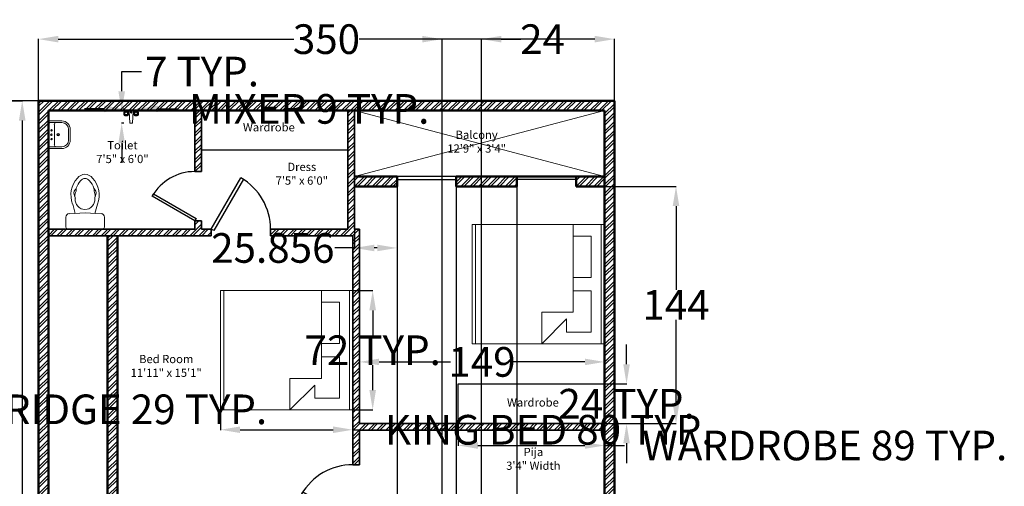
# Model space of a CAD drawing. Units: inches. Extents: x 73 to 1216, y -495 to 328.
# Tile 9 of 9: x 569 to 1167, y 45 to 328. Entities that reach past the tile are written whole.
import ezdxf

# ---------------------------------------------------------------- set-up
doc = ezdxf.new("R2010")
doc.units = ezdxf.units.IN
for name, color, linetype, lineweight in [('A-ANNO-DIMS', 2, 'Continuous', 18), ('A-AREA-IDEN', 7, 'Continuous', 18), ('A-DOOR', 3, 'Continuous', 25), ('A-FLOR-CASE', 2, 'Continuous', 25), ('A-FLOR-FIXT', 9, 'Continuous', 18), ('A-FLOR-OPEN', 8, 'Continuous', 13), ('A-WALL-PATT', 8, 'Continuous', 13), ('Furniture', 2, 'Continuous', 18), ('Inner Walls', 5, 'Continuous', 35), ('Outer Walls', 1, 'Continuous', 50), ('Text-T18', 7, 'Continuous', 18)]:
    doc.layers.add(name, color=color, linetype=linetype, lineweight=lineweight)
doc.styles.get("Standard").update_dxf_attribs({"font": 'arial.ttf'})
doc.dimstyles.get("Standard").update_dxf_attribs({"dimtxt": 18, "dimasz": 12, "dimexe": 0.18, "dimexo": 0.0625, "dimgap": 0.09, "dimtad": 0, "dimtih": 1, "dimtoh": 1, "dimdec": 0, "dimzin": 0, "dimdsep": 46, "dimlunit": 3, "dimtxsty": 'Standard', "dimcen": 0.09, "dimadec": 0, "dimazin": 0, "dimtfac": 1, "dimtdec": 0, "dimtofl": 0, "dimtmove": 0, "dimatfit": 3, "dimfxl": 1, "dimtolj": 1, "dimtzin": 0, "dimarcsym": 0})
pattern_1 = [(45, (-647.324, -1257.0093), (-2.694077, 2.694077), []), (45, (-645.528, -1257.0093), (-2.694077, 2.694077), [])]

# ---------------------------------------------------------------- blocks, each defined once
blk = doc.blocks.new('*U2')
for p, q in [((0, 0), (0, -4)), ((36, 0), (36, -4))]:
    blk.add_line(p, q)
blk.add_lwpolyline([(0, 0), (18, 31.18), (19.52, 30.3), (1.52, -0.88)], close=True)
blk.add_arc((0, 0), 36, 0, 60)
blk = doc.blocks.new('*U3')
for p, q in [((0, 0), (0, -4)), ((30, 0), (30, -4))]:
    blk.add_line(p, q)
blk.add_lwpolyline([(0, 0), (15, 25.98), (16.52, 25.11), (1.52, -0.88)], close=True)
blk.add_arc((0, 0), 30, 0, 60)
blk = doc.blocks.new('*U21')
for p, q in [((0, 0), (0, -6)), ((36, 0), (36, -6))]:
    blk.add_line(p, q)
blk.add_lwpolyline([(0, 0), (36, 0), (36, -1.75), (0, -1.75)], close=True)
blk = doc.blocks.new('KING-00')
for p, q in [((-0.897, -0.947), (-0.897, 0.882)), ((0.602, 0.882), (0.602, -0.464)), ((1.034, -0.947), (1.034, 0.882)), ((0.602, 0.704), (0.881, 0.704)), ((0.881, 0.069), (0.881, 0.704)), ((0.602, 0.069), (0.881, 0.069)), ((0.881, -0.134), (0.602, -0.134)), ((0.881, -0.769), (0.881, -0.134)), ((0.119, -0.464), (0.119, -0.947)), ((0.602, -0.464), (0.119, -0.464)), ((0.119, -0.947), (0.5, -0.566)), ((0.5, -0.769), (0.5, -0.566)), ((0.5, -0.769), (0.881, -0.769))]:
    blk.add_line(p, q)
blk.add_lwpolyline([(-0.948, -0.947), (-0.948, 0.882), (1.084, 0.882), (1.084, -0.947)], close=True)
blk = doc.blocks.new('A$C1308471B')
at = {"ltscale": 20}
for p, q in [((0, 0.461), (0, 0.019)), ((0.035, 0.479), (0.15, 0.479)), ((0.201, 0.24), (0.192, 0.438)), ((0.196, 0.364), (0.311, 0.395)), ((0.498, 0.357), (0.482, 0.371)), ((0.502, 0.353), (0.472, 0.353)), ((0.201, 0.24), (0.192, 0.041)), ((0.502, 0.13), (0.472, 0.13)), ((0.498, 0.126), (0.482, 0.112)), ((0.035, 0), (0.15, 0)), ((0.196, 0.119), (0.311, 0.088))]:
    blk.add_line(p, q, dxfattribs=at)
for centre, radius, start, end in [((0.006, 0.461), 0.006, 136.5269, 180), ((0.035, 0.433), 0.0465, 90, 136.5269), ((0.15, 0.436), 0.0429, 2.5755, 90), ((0.425, 0.11), 0.307, 47.4135, 111.7924), ((0.449, 0.264), 0.115, 79.3968, 118.5742), ((0.405, 0.216), 0.153, 63.502, 90.4522), ((0.466, 0.351), 0.0255, 50, 79.3968), ((0.365, 0.242), 0.121, 83.3523, 180), ((0.382, 0.387), 0.0255, 263.3523, 298.5742), ((0.515, 0.377), 0.0255, 230, 251.3881), ((0.502, 0.327), 0.0255, 70.3751, 90), ((0.425, 0.11), 0.256, 46.612, 70.3751), ((0.565, 0.242), 0.065, 0, 57.2974), ((0.565, 0.242), 0.116, 0, 54.7115), ((0.365, 0.242), 0.121, 180, 276.6477), ((0.425, 0.373), 0.307, 248.2076, 312.5865), ((0.405, 0.267), 0.153, 269.5478, 296.498), ((0.515, 0.106), 0.0255, 108.6119, 130), ((0.502, 0.156), 0.0255, 270, 289.6249), ((0.425, 0.373), 0.256, 289.6249, 313.388), ((0.565, 0.242), 0.065, 302.7026, 0), ((0.565, 0.242), 0.116, 305.2885, 0), ((0.006, 0.019), 0.006, 180, 223.4731), ((0.035, 0.047), 0.0465, 223.4731, 270), ((0.15, 0.043), 0.0429, 270, 357.4245), ((0.382, 0.096), 0.0255, 61.4258, 96.6477), ((0.449, 0.22), 0.115, 241.4258, 280.6032), ((0.466, 0.132), 0.0255, 280.6032, 310)]:
    blk.add_arc(centre, radius, start, end, dxfattribs=at)
blk = doc.blocks.new('A$C57EA129C')
for p, q in [((0, 0.443), (0, 0.178)), ((0.016, 0.459), (0.563, 0.459)), ((0.036, 0.432), (0.036, 0.29)), ((0.045, 0.441), (0.535, 0.441)), ((0.544, 0.432), (0.544, 0.29)), ((0.579, 0.443), (0.579, 0.178)), ((0.036, 0.29), (0.036, 0.178)), ((0.08, 0.334), (0.499, 0.334)), ((0.544, 0.29), (0.544, 0.178)), ((0.178, 0.036), (0.401, 0.036)), ((0.178, 0), (0.401, 0))]:
    blk.add_line(p, q)
for centre, radius in [((0.198, 0.392), 0.0143), ((0.29, 0.255), 0.0267), ((0.29, 0.255), 0.0178), ((0.29, 0.396), 0.0156), ((0.381, 0.392), 0.0143)]:
    blk.add_circle(centre, radius)
for centre, radius, start, end in [((0.016, 0.443), 0.016, 90, 180), ((0.045, 0.432), 0.00891, 90, 180), ((0.535, 0.432), 0.00891, 0, 90), ((0.563, 0.443), 0.016, 0, 90), ((0.08, 0.29), 0.0445, 90, 180), ((0.499, 0.29), 0.0445, 0, 90), ((0.178, 0.178), 0.178, 180, 270), ((0.178, 0.178), 0.143, 180, 270), ((0.401, 0.178), 0.178, 270, 0), ((0.401, 0.178), 0.143, 270, 0)]:
    blk.add_arc(centre, radius, start, end)
blk = doc.blocks.new('A$C68D75330')
for p, q in [((0.155, 0.406), (0.155, 0.451)), ((0.167, 0.404), (0.167, 0.454)), ((0.172, 0.459), (0.222, 0.459)), ((0.222, 0.399), (0.172, 0.399)), ((0.175, 0.471), (0.22, 0.471)), ((0.22, 0.386), (0.175, 0.386)), ((0.227, 0.454), (0.227, 0.404)), ((0.24, 0.451), (0.24, 0.406)), ((0.264, 0.256), (0.252, 0.461)), ((0.275, 0.471), (0.305, 0.471)), ((0.327, 0.461), (0.315, 0.256)), ((0.34, 0.451), (0.34, 0.406)), ((0.352, 0.454), (0.352, 0.404)), ((0.407, 0.459), (0.357, 0.459)), ((0.357, 0.399), (0.407, 0.399)), ((0.405, 0.471), (0.36, 0.471)), ((0.36, 0.386), (0.405, 0.386)), ((0.412, 0.404), (0.412, 0.454)), ((0.425, 0.406), (0.425, 0.451)), ((0.306, 0.246), (0.274, 0.246))]:
    blk.add_line(p, q)
for centre, radius in [((0.197, 0.429), 0.03), ((0.197, 0.429), 0.0232), ((0.29, 0.446), 0.0125), ((0.29, 0.446), 0.00625), ((0.382, 0.429), 0.03), ((0.382, 0.429), 0.0232)]:
    blk.add_circle(centre, radius)
for centre, radius, start, end in [((0.175, 0.451), 0.02, 90, 180), ((0.175, 0.406), 0.02, 180, 270), ((0.172, 0.454), 0.005, 90, 180), ((0.172, 0.404), 0.005, 180, 270), ((0.22, 0.451), 0.02, 0, 90), ((0.22, 0.406), 0.02, 270, 0), ((0.222, 0.454), 0.005, 0, 90), ((0.222, 0.404), 0.005, 270, 0), ((0.274, 0.444), 0.0273, 87.1975, 140.7274), ((0.306, 0.444), 0.0273, 39.2726, 92.8025), ((0.36, 0.451), 0.02, 90, 180), ((0.36, 0.406), 0.02, 180, 270), ((0.357, 0.454), 0.005, 90, 180), ((0.357, 0.404), 0.005, 180, 270), ((0.405, 0.451), 0.02, 0, 90), ((0.405, 0.406), 0.02, 270, 0), ((0.407, 0.454), 0.005, 0, 90), ((0.407, 0.404), 0.005, 270, 0), ((0.274, 0.256), 0.01, 183.3274, 270), ((0.306, 0.256), 0.01, 270, 356.6726)]:
    blk.add_arc(centre, radius, start, end)
blk = doc.blocks.new('WARDROBE-89X24')
blk.add_lwpolyline([(0, 24), (89, 24), (89, 0), (0, 0)], close=True)
blk = doc.blocks.new('*D26')
at = {"layer": 'A-ANNO-DIMS', "color": 0, "lineweight": -2, "transparency": 16777216}
for p, q in [((690.69, 91.4), (690.69, 79.21)), ((771.16, 91.4), (771.16, 79.21)), ((702.69, 79.39), (759.16, 79.39)), ((771.16, 79.39), (783.16, 79.39))]:
    blk.add_line(p, q, dxfattribs=at)
at = {"layer": 'A-ANNO-DIMS', "color": 0, "transparency": 16777216}
for points in [[(702.69, 81.39), (702.69, 77.39), (690.69, 79.39)], [(759.16, 81.39), (759.16, 77.39), (771.16, 79.39)]]:
    blk.add_solid(points, dxfattribs=at)
at = {"layer": 'Defpoints', "color": 0, "transparency": 16777216}
for p in [(690.69, 91.46), (771.16, 91.46), (771.16, 79.39)]:
    blk.add_point(p, dxfattribs=at)
at = {"layer": 'A-ANNO-DIMS', "color": 0, "transparency": 16777216, "insert": (890.24, 79.39), "char_height": 18, "attachment_point": 5}
blk.add_mtext('\\A1;KING BED 80 TYP.', dxfattribs=at)
blk = doc.blocks.new('*D27')
at = {"layer": 'A-ANNO-DIMS', "color": 0, "lineweight": -2, "transparency": 16777216}
for p, q in [((771.23, 163.89), (783.42, 163.89)), ((783.24, 151.89), (783.24, 136.81)), ((783.24, 103.46), (783.24, 118.54)), ((771.23, 91.46), (783.42, 91.46))]:
    blk.add_line(p, q, dxfattribs=at)
at = {"layer": 'A-ANNO-DIMS', "color": 0, "transparency": 16777216}
for points in [[(781.24, 151.89), (785.24, 151.89), (783.24, 163.89)], [(781.24, 103.46), (785.24, 103.46), (783.24, 91.46)]]:
    blk.add_solid(points, dxfattribs=at)
at = {"layer": 'Defpoints', "color": 0, "transparency": 16777216}
for p in [(771.16, 163.89), (783.24, 163.89), (771.16, 91.46)]:
    blk.add_point(p, dxfattribs=at)
at = {"layer": 'A-ANNO-DIMS', "color": 0, "transparency": 16777216, "insert": (783.24, 127.68), "char_height": 18, "attachment_point": 5}
blk.add_mtext('\\A1;72 TYP.', dxfattribs=at)
blk = doc.blocks.new('*D34')
at = {"layer": 'A-ANNO-DIMS', "color": 0, "lineweight": -2, "transparency": 16777216}
for p, q in [((620.04, 274.23), (608.04, 274.23)), ((632.04, 272.97), (632.04, 274.41)), ((640.86, 272.97), (640.86, 274.41)), ((652.86, 274.23), (664.86, 274.23))]:
    blk.add_line(p, q, dxfattribs=at)
at = {"layer": 'A-ANNO-DIMS', "color": 0, "transparency": 16777216}
for points in [[(620.04, 276.23), (620.04, 272.23), (632.04, 274.23)], [(652.86, 276.23), (652.86, 272.23), (640.86, 274.23)]]:
    blk.add_solid(points, dxfattribs=at)
at = {"layer": 'Defpoints', "color": 0, "transparency": 16777216}
for p in [(632.04, 272.9), (640.86, 274.23), (640.86, 272.9)]:
    blk.add_point(p, dxfattribs=at)
at = {"layer": 'A-ANNO-DIMS', "color": 0, "transparency": 16777216, "insert": (744.67, 274.23), "char_height": 18, "attachment_point": 5}
blk.add_mtext('\\A1;MIXER 9 TYP.', dxfattribs=at)
blk = doc.blocks.new('*D35')
at = {"layer": 'A-ANNO-DIMS', "color": 0, "lineweight": -2, "transparency": 16777216}
for p, q in [((630.72, 284.9), (630.72, 296.9)), ((630.72, 296.9), (642.72, 296.9)), ((631.98, 272.9), (630.54, 272.9)), ((631.98, 265.54), (630.54, 265.54)), ((630.72, 253.54), (630.72, 241.54))]:
    blk.add_line(p, q, dxfattribs=at)
at = {"layer": 'A-ANNO-DIMS', "color": 0, "transparency": 16777216}
for points in [[(628.72, 284.9), (632.72, 284.9), (630.72, 272.9)], [(628.72, 253.54), (632.72, 253.54), (630.72, 265.54)]]:
    blk.add_solid(points, dxfattribs=at)
at = {"layer": 'Defpoints', "color": 0, "transparency": 16777216}
for p in [(630.72, 272.9), (632.04, 272.9), (632.04, 265.54)]:
    blk.add_point(p, dxfattribs=at)
at = {"layer": 'A-ANNO-DIMS', "color": 0, "transparency": 16777216, "insert": (679.55, 296.9), "char_height": 18, "attachment_point": 5}
blk.add_mtext('\\A1;7 TYP.', dxfattribs=at)
blk = doc.blocks.new('*D38')
at = {"layer": 'A-ANNO-DIMS', "color": 0, "lineweight": -2, "transparency": 16777216}
for p, q in [((835.16, 83.11), (835.16, 69.65)), ((924.16, 83.11), (924.16, 69.65)), ((847.16, 69.83), (912.16, 69.83)), ((924.16, 69.83), (936.16, 69.83))]:
    blk.add_line(p, q, dxfattribs=at)
at = {"layer": 'A-ANNO-DIMS', "color": 0, "transparency": 16777216}
for points in [[(847.16, 71.83), (847.16, 67.83), (835.16, 69.83)], [(912.16, 71.83), (912.16, 67.83), (924.16, 69.83)]]:
    blk.add_solid(points, dxfattribs=at)
at = {"layer": 'Defpoints', "color": 0, "transparency": 16777216}
for p in [(835.16, 83.18), (924.16, 83.18), (924.16, 69.83)]:
    blk.add_point(p, dxfattribs=at)
at = {"layer": 'A-ANNO-DIMS', "color": 0, "transparency": 16777216, "insert": (1057.97, 69.83), "char_height": 18, "attachment_point": 5}
blk.add_mtext('\\A1;WARDROBE 89 TYP.', dxfattribs=at)
blk = doc.blocks.new('*D39')
at = {"layer": 'A-ANNO-DIMS', "color": 0, "lineweight": -2, "transparency": 16777216}
for p, q in [((937.51, 119.18), (937.51, 131.18)), ((924.23, 107.18), (937.69, 107.18)), ((924.23, 83.18), (937.69, 83.18)), ((937.51, 71.18), (937.51, 59.18))]:
    blk.add_line(p, q, dxfattribs=at)
at = {"layer": 'A-ANNO-DIMS', "color": 0, "transparency": 16777216}
for points in [[(935.51, 119.18), (939.51, 119.18), (937.51, 107.18)], [(935.51, 71.18), (939.51, 71.18), (937.51, 83.18)]]:
    blk.add_solid(points, dxfattribs=at)
at = {"layer": 'Defpoints', "color": 0, "transparency": 16777216}
for p in [(924.16, 107.18), (937.51, 107.18), (924.16, 83.18)]:
    blk.add_point(p, dxfattribs=at)
at = {"layer": 'A-ANNO-DIMS', "color": 0, "transparency": 16777216, "insert": (937.51, 95.18), "char_height": 18, "attachment_point": 5}
blk.add_mtext('\\A1;24 TYP.', dxfattribs=at)
blk = doc.blocks.new('*D40')
at = {"layer": 'A-ANNO-DIMS', "color": 0, "lineweight": -2, "transparency": 16777216}
for p, q in [((497.66, 96.03), (497.66, 91.62)), ((526.23, 96.03), (526.23, 91.62)), ((509.66, 91.8), (514.23, 91.8)), ((526.23, 91.8), (538.23, 91.8))]:
    blk.add_line(p, q, dxfattribs=at)
at = {"layer": 'A-ANNO-DIMS', "color": 0, "transparency": 16777216}
for points in [[(509.66, 93.8), (509.66, 89.8), (497.66, 91.8)], [(514.23, 93.8), (514.23, 89.8), (526.23, 91.8)]]:
    blk.add_solid(points, dxfattribs=at)
at = {"layer": 'Defpoints', "color": 0, "transparency": 16777216}
for p in [(497.66, 96.09), (526.23, 96.09), (526.23, 91.8)]:
    blk.add_point(p, dxfattribs=at)
at = {"layer": 'A-ANNO-DIMS', "color": 0, "transparency": 16777216, "insert": (632.61, 91.8), "char_height": 18, "attachment_point": 5}
blk.add_mtext('\\A1;FRIDGE 29 TYP.', dxfattribs=at)
blk = doc.blocks.new('*D51')
at = {"layer": 'A-ANNO-DIMS', "color": 0, "lineweight": -2, "transparency": 16777216}
for p, q in [((532.94, 279.18), (570.45, 279.18)), ((570.27, 267.18), (570.27, -65.04)), ((570.27, -415.82), (570.27, -83.6)), ((532.94, -427.82), (570.45, -427.82))]:
    blk.add_line(p, q, dxfattribs=at)
at = {"layer": 'A-ANNO-DIMS', "color": 0, "transparency": 16777216}
for points in [[(568.27, 267.18), (572.27, 267.18), (570.27, 279.18)], [(568.27, -415.82), (572.27, -415.82), (570.27, -427.82)]]:
    blk.add_solid(points, dxfattribs=at)
at = {"layer": 'Defpoints', "color": 0, "transparency": 16777216}
for p in [(532.87, 279.18), (570.27, 279.18), (532.87, -427.82)]:
    blk.add_point(p, dxfattribs=at)
at = {"layer": 'A-ANNO-DIMS', "color": 0, "transparency": 16777216, "insert": (570.27, -74.32), "char_height": 18, "attachment_point": 5}
blk.add_mtext('\\A1;707', dxfattribs=at)
blk = doc.blocks.new('*D52')
at = {"layer": 'A-ANNO-DIMS', "color": 0, "lineweight": -2, "transparency": 16777216}
for p, q in [((580.16, 279.24), (580.16, 316.76)), ((592.16, 316.58), (735.23, 316.58)), ((918.16, 316.58), (775.1, 316.58)), ((930.16, 279.24), (930.16, 316.76))]:
    blk.add_line(p, q, dxfattribs=at)
at = {"layer": 'A-ANNO-DIMS', "color": 0, "transparency": 16777216}
for points in [[(592.16, 318.58), (592.16, 314.58), (580.16, 316.58)], [(918.16, 318.58), (918.16, 314.58), (930.16, 316.58)]]:
    blk.add_solid(points, dxfattribs=at)
at = {"layer": 'Defpoints', "color": 0, "transparency": 16777216}
for p in [(930.16, 316.58), (580.16, 279.18), (930.16, 279.18)]:
    blk.add_point(p, dxfattribs=at)
at = {"layer": 'A-ANNO-DIMS', "color": 0, "transparency": 16777216, "insert": (755.16, 316.58), "char_height": 18, "attachment_point": 5}
blk.add_mtext('\\A1;350', dxfattribs=at)
blk = doc.blocks.new('*D53')
at = {"layer": 'A-ANNO-DIMS', "color": 0, "lineweight": -2, "transparency": 16777216}
for p, q in [((580.1, 279.18), (542.58, 279.18)), ((542.76, 267.18), (542.76, -65.04)), ((542.76, -415.82), (542.76, -83.6)), ((580.1, -427.82), (542.58, -427.82))]:
    blk.add_line(p, q, dxfattribs=at)
at = {"layer": 'A-ANNO-DIMS', "color": 0, "transparency": 16777216}
for points in [[(540.76, 267.18), (544.76, 267.18), (542.76, 279.18)], [(540.76, -415.82), (544.76, -415.82), (542.76, -427.82)]]:
    blk.add_solid(points, dxfattribs=at)
at = {"layer": 'Defpoints', "color": 0, "transparency": 16777216}
for p in [(542.76, 279.18), (580.16, 279.18), (580.16, -427.82)]:
    blk.add_point(p, dxfattribs=at)
at = {"layer": 'A-ANNO-DIMS', "color": 0, "transparency": 16777216, "insert": (542.76, -74.32), "char_height": 18, "attachment_point": 5}
blk.add_mtext('\\A1;707', dxfattribs=at)
blk = doc.blocks.new('*D57')
at = {"layer": 'A-ANNO-DIMS', "color": 0, "lineweight": -2, "transparency": 16777216}
for p, q in [((775.16, 83.24), (775.16, 120.76)), ((787.16, 120.58), (830.52, 120.58)), ((912.16, 120.58), (868.81, 120.58)), ((924.16, 83.24), (924.16, 120.76))]:
    blk.add_line(p, q, dxfattribs=at)
at = {"layer": 'A-ANNO-DIMS', "color": 0, "transparency": 16777216}
for points in [[(787.16, 122.58), (787.16, 118.58), (775.16, 120.58)], [(912.16, 122.58), (912.16, 118.58), (924.16, 120.58)]]:
    blk.add_solid(points, dxfattribs=at)
at = {"layer": 'Defpoints', "color": 0, "transparency": 16777216}
for p in [(924.16, 120.58), (775.16, 83.18), (924.16, 83.18)]:
    blk.add_point(p, dxfattribs=at)
at = {"layer": 'A-ANNO-DIMS', "color": 0, "transparency": 16777216, "insert": (849.66, 120.58), "char_height": 18, "attachment_point": 5}
blk.add_mtext('\\A1;149', dxfattribs=at)
blk = doc.blocks.new('*D58')
at = {"layer": 'A-ANNO-DIMS', "color": 0, "lineweight": -2, "transparency": 16777216}
for p, q in [((924.23, 227.18), (967.74, 227.18)), ((967.56, 215.18), (967.56, 164.3)), ((967.56, 95.18), (967.56, 146.05)), ((924.23, 83.18), (967.74, 83.18))]:
    blk.add_line(p, q, dxfattribs=at)
at = {"layer": 'A-ANNO-DIMS', "color": 0, "transparency": 16777216}
for points in [[(965.56, 215.18), (969.56, 215.18), (967.56, 227.18)], [(965.56, 95.18), (969.56, 95.18), (967.56, 83.18)]]:
    blk.add_solid(points, dxfattribs=at)
at = {"layer": 'Defpoints', "color": 0, "transparency": 16777216}
for p in [(924.16, 227.18), (967.56, 227.18), (924.16, 83.18)]:
    blk.add_point(p, dxfattribs=at)
at = {"layer": 'A-ANNO-DIMS', "color": 0, "transparency": 16777216, "insert": (967.56, 155.18), "char_height": 18, "attachment_point": 5}
blk.add_mtext('\\A1;144', dxfattribs=at)
blk = doc.blocks.new('*D67')
at = {"layer": 'A-ANNO-DIMS', "color": 0, "lineweight": -2, "transparency": 16777216}
for p, q in [((798.02113, 227.113801), (798.02113, -465.403699)), ((834.02113, 227.113801), (834.02113, -465.403699)), ((786.02113, -465.223699), (774.02113, -465.223699)), ((846.02113, -465.223699), (858.02113, -465.223699))]:
    blk.add_line(p, q, dxfattribs=at)
at = {"layer": 'A-ANNO-DIMS', "color": 0, "transparency": 16777216}
for points in [[(786.02113, -463.223699), (786.02113, -467.223699), (798.02113, -465.223699)], [(846.02113, -463.223699), (846.02113, -467.223699), (834.02113, -465.223699)]]:
    blk.add_solid(points, dxfattribs=at)
at = {"layer": 'Defpoints', "color": 0, "transparency": 16777216}
for p in [(798.02113, 227.176301), (834.02113, 227.176301), (834.02113, -465.223699)]:
    blk.add_point(p, dxfattribs=at)
at = {"layer": 'A-ANNO-DIMS', "color": 0, "transparency": 16777216, "insert": (816.02113, -465.223699), "char_height": 18, "attachment_point": 5}
blk.add_mtext('\\A1;36', dxfattribs=at)
blk = doc.blocks.new('*D68')
at = {"layer": 'A-ANNO-DIMS', "color": 0, "lineweight": -2, "transparency": 16777216}
for p, q in [((834.02, 227.11), (834.02, -465.4)), ((870.82, 227.11), (870.82, -465.4)), ((846.02, -465.22), (858.82, -465.22)), ((870.82, -465.22), (882.82, -465.22))]:
    blk.add_line(p, q, dxfattribs=at)
at = {"layer": 'A-ANNO-DIMS', "color": 0, "transparency": 16777216}
for points in [[(846.02, -463.22), (846.02, -467.22), (834.02, -465.22)], [(858.82, -463.22), (858.82, -467.22), (870.82, -465.22)]]:
    blk.add_solid(points, dxfattribs=at)
at = {"layer": 'Defpoints', "color": 0, "transparency": 16777216}
for p in [(834.02, 227.18), (870.82, 227.18), (870.82, -465.22)]:
    blk.add_point(p, dxfattribs=at)
at = {"layer": 'A-ANNO-DIMS', "color": 0, "transparency": 16777216, "insert": (906.3, -465.22), "char_height": 18, "attachment_point": 5}
blk.add_mtext('\\A1;36.8', dxfattribs=at)
blk = doc.blocks.new('*D69')
at = {"layer": 'A-ANNO-DIMS', "color": 0, "lineweight": -2, "transparency": 16777216}
for p, q in [((772.16, 227.11), (772.16, 189.6)), ((798.02, 227.11), (798.02, 189.6)), ((772.16, 189.78), (760.16, 189.78)), ((786.02, 189.78), (784.16, 189.78))]:
    blk.add_line(p, q, dxfattribs=at)
at = {"layer": 'A-ANNO-DIMS', "color": 0, "transparency": 16777216}
for points in [[(784.16, 191.78), (784.16, 187.78), (772.16, 189.78)], [(786.02, 191.78), (786.02, 187.78), (798.02, 189.78)]]:
    blk.add_solid(points, dxfattribs=at)
at = {"layer": 'Defpoints', "color": 0, "transparency": 16777216}
for p in [(772.16, 227.18), (798.02, 227.18), (772.16, 189.78)]:
    blk.add_point(p, dxfattribs=at)
at = {"layer": 'A-ANNO-DIMS', "color": 0, "transparency": 16777216, "insert": (722.56, 189.78), "char_height": 18, "attachment_point": 5}
blk.add_mtext('\\A1;25.856', dxfattribs=at)
blk = doc.blocks.new('*D77')
at = {"layer": 'A-ANNO-DIMS', "color": 0, "lineweight": -2, "transparency": 16777216}
for p, q in [((813.36, 316.58), (801.36, 316.58)), ((825.36, -180.08), (825.36, 316.76)), ((849.36, -180.08), (849.36, 316.76)), ((861.36, 316.58), (873.36, 316.58))]:
    blk.add_line(p, q, dxfattribs=at)
at = {"layer": 'A-ANNO-DIMS', "color": 0, "transparency": 16777216}
for points in [[(813.36, 318.58), (813.36, 314.58), (825.36, 316.58)], [(861.36, 318.58), (861.36, 314.58), (849.36, 316.58)]]:
    blk.add_solid(points, dxfattribs=at)
at = {"layer": 'Defpoints', "color": 0, "transparency": 16777216}
for p in [(849.36, 316.58), (825.36, -180.14), (849.36, -180.14)]:
    blk.add_point(p, dxfattribs=at)
at = {"layer": 'A-ANNO-DIMS', "color": 0, "transparency": 16777216, "insert": (886.46, 316.58), "char_height": 18, "attachment_point": 5}
blk.add_mtext('\\A1;24', dxfattribs=at)

msp = doc.modelspace()

# ---------------------------------------------------------------- hatches: boundary and pattern name
at = {"layer": 'A-WALL-PATT'}
h = msp.add_hatch(dxfattribs=at)
h.set_pattern_fill('ANSI32', color=256, scale=0.4)
h.set_pattern_definition(pattern_1)
h.paths.add_polyline_path([(586.1647, 273.1763), (924.1647, 273.1763), (924.1647, -421.8237), (753.1647, -421.8237), (753.1647, -427.8237), (930.1647, -427.8237), (930.1647, 279.1763), (580.1647, 279.1763), (580.1647, -427.8237), (633.1647, -427.8237), (633.1647, -421.8237), (586.1647, -421.8237)])
h = msp.add_hatch(dxfattribs=at)
h.set_pattern_fill('ANSI32', color=256, scale=0.4)
h.set_pattern_definition(pattern_1)
h.paths.add_polyline_path([(685.1647, 201.1763), (679.1647, 201.1763), (679.1647, 206.1763), (675.1647, 206.1763), (675.1647, 201.1763), (586.1647, 201.1763), (586.1647, 197.1763), (685.1647, 197.1763)])
h.paths.add_polyline_path([(679.1647, 273.1763), (675.1647, 273.1763), (675.1647, 236.1763), (679.1647, 236.1763)])
h.paths.add_polyline_path([(775.1647, 201.1763), (772.1647, 201.1763), (772.1647, 273.1763), (768.1647, 273.1763), (768.1647, 249.1763), (768.1647, 201.1763), (721.1647, 201.1763), (721.1647, 197.1763), (771.1647, 197.1763), (771.1647, 58.1763), (775.1647, 58.1763)])
h.paths.add_polyline_path([(798.0211, 233.1763), (772.1647, 233.1763), (772.1647, 227.1763), (798.0211, 227.1763)])
h.paths.add_polyline_path([(870.8232, 233.1763), (834.0211, 233.1763), (834.0211, 227.1763), (870.8232, 227.1763)])
h.paths.add_polyline_path([(924.1647, 233.1763), (906.8232, 233.1763), (906.8232, 227.1763), (924.1647, 227.1763)])
h.paths.add_polyline_path([(924.1647, 83.1763), (775.1647, 83.1763), (775.1647, 79.1763), (924.1647, 79.1763)])
h.paths.add_polyline_path([(775.1647, 22.1763), (771.1647, 22.1763), (771.1647, 16.1763), (628.1647, 16.1763), (628.1647, 12.1763), (775.1647, 12.1763)])
h.paths.add_polyline_path([(692.1647, 12.1763), (688.1647, 12.1763), (688.1647, -52.8237), (692.1647, -52.8237)])
h.paths.add_polyline_path([(924.1647, 39.1763), (824.1647, 39.1763), (824.1647, 35.1763), (924.1647, 35.1763)])
h.paths.add_polyline_path([(874.6647, -29.8237), (864.1647, -29.8237), (824.1647, -29.8237), (824.1647, -87.8237), (817.1647, -87.8237), (817.1647, -91.8237), (844.6647, -91.8237), (844.6647, -87.8237), (828.1647, -87.8237), (828.1647, -33.8237), (874.6647, -33.8237)])
h.paths.add_polyline_path([(924.1647, -29.8237), (910.6647, -29.8237), (910.6647, -33.8237), (924.1647, -33.8237)])
h.paths.add_polyline_path([(924.1647, -87.8237), (904.6647, -87.8237), (904.6647, -91.8237), (924.1647, -91.8237)])
h.paths.add_polyline_path([(777.1647, -88.8237), (761.1647, -88.8237), (761.1647, -92.8237), (767.1647, -92.8237), (767.1647, -224.8237), (771.1647, -224.8237), (771.1647, -92.8237), (777.1647, -92.8237)])
h.paths.add_polyline_path([(725.1647, -88.8237), (628.1647, -88.8237), (628.1647, -92.8237), (725.1647, -92.8237)])
h.paths.add_polyline_path([(692.1647, -82.8237), (688.1647, -82.8237), (688.1647, -88.8237), (692.1647, -88.8237)])
h.paths.add_polyline_path([(767.1647, -313.8237), (924.1647, -313.8237), (924.1647, -307.8237), (763.1647, -307.8237), (763.1647, -421.8237), (767.1647, -421.8237)])
h = msp.add_hatch(dxfattribs=at)
h.set_pattern_fill('ANSI32', color=256, scale=0.4)
h.set_pattern_definition(pattern_1)
h.paths.add_polyline_path([(628.1647, 197.1763), (622.1647, 197.1763), (622.1647, -230.8237), (771.1647, -230.8237), (771.1647, -224.8237), (628.1647, -224.8237)])

# ---------------------------------------------------------------- linework, layer by layer
at = {"layer": 'A-FLOR-OPEN'}
for p, q in [((924.1647, 233.1763), (772.1647, 273.1763)), ((772.1647, 233.1763), (924.1647, 273.1763))]:
    msp.add_line(p, q, dxfattribs=at)
at = {"layer": 'Inner Walls'}
for p, q in [((675.1647, 273.1763), (675.1647, 236.1763)), ((679.1647, 273.1763), (679.1647, 236.1763)), ((768.1647, 273.1763), (768.1647, 201.1763)), ((772.1647, 273.1763), (772.1647, 201.1763)), ((675.1647, 236.1763), (679.1647, 236.1763)), ((675.1647, 206.1763), (675.1647, 201.1763)), ((679.1647, 206.1763), (675.1647, 206.1763)), ((679.1647, 206.1763), (679.1647, 201.1763)), ((675.1647, 201.1763), (586.1647, 201.1763)), ((685.1647, 201.1763), (679.1647, 201.1763)), ((685.1647, 201.1763), (685.1647, 197.1763)), ((768.1647, 201.1763), (721.1647, 201.1763)), ((721.1647, 197.1763), (721.1647, 201.1763)), ((772.1647, 201.1763), (775.1647, 201.1763)), ((775.1647, 201.1763), (775.1647, 83.1763)), ((685.1647, 197.1763), (586.1647, 197.1763)), ((771.1647, 197.1763), (721.1647, 197.1763)), ((771.1647, 197.1763), (771.1647, 58.1763)), ((775.1647, 83.1763), (924.1647, 83.1763)), ((775.1647, 79.1763), (924.1647, 79.1763)), ((775.1647, 79.1763), (775.1647, 58.1763)), ((775.1647, 58.1763), (771.1647, 58.1763))]:
    msp.add_line(p, q, dxfattribs=at)
at = {"layer": 'Outer Walls'}
for p, q in [((580.1647, 279.1763), (930.1647, 279.1763)), ((580.1647, -427.8237), (580.1647, 279.1763)), ((930.1647, -427.8237), (930.1647, 279.1763)), ((586.1647, 273.1763), (924.1647, 273.1763)), ((586.1647, -421.8237), (586.1647, 273.1763)), ((924.1647, -421.8237), (924.1647, 273.1763)), ((772.1647, 233.1763), (798.0211, 233.1763)), ((798.0211, 233.1763), (798.0211, 227.1763)), ((834.0211, 233.1763), (924.1647, 233.1763)), ((834.0211, 233.1763), (834.0211, 227.1763)), ((870.8232, 233.1763), (870.8232, 227.1763)), ((906.8232, 233.1763), (906.8232, 227.1763)), ((772.1647, 227.1763), (798.0211, 227.1763)), ((834.0211, 227.1763), (870.8232, 227.1763)), ((906.8232, 227.1763), (924.1647, 227.1763)), ((622.1647, -230.8237), (622.1647, 197.1763)), ((628.1647, -224.8237), (628.1647, 197.1763))]:
    msp.add_line(p, q, dxfattribs=at)

# ---------------------------------------------------------------- block references
at = {"layer": 'A-DOOR', "rotation": 90}
for name, p in [('*U3', (675.1647, 206.1763)), ('*U2', (771.1647, 22.1763))]:
    msp.add_blockref(name, p, dxfattribs=at)
at = {"layer": 'A-DOOR'}
for name, p in [('*U2', (685.1647, 201.1763)), ('*U21', (870.8232, 233.1763))]:
    msp.add_blockref(name, p, dxfattribs=at)
at = {"layer": 'A-DOOR', "xscale": -1}
msp.add_blockref('*U21', (834.0211, 233.1763), dxfattribs=at)
at = {"layer": 'A-FLOR-CASE'}
for p in [(679.1651, 249.176), (835.1651, 83.176)]:
    msp.add_blockref('WARDROBE-89X24', p, dxfattribs=at)
at = {"layer": 'A-FLOR-FIXT', "xscale": 32.67217261962217, "yscale": 32.67217261962217, "zscale": 32.67217261962217}
msp.add_blockref('A$C68D75330', (626.9766, 257.4873), dxfattribs=at)
at = {"layer": 'A-FLOR-FIXT'}
for name, p, xscale, yscale, zscale, rotation in [('A$C57EA129C', (599.4641, 266.948), -28.98333223671166, 28.98333223671166, 28.98333223671166, 90), ('A$C1308471B', (620.2612, 201.1763), 48.95497407897215, 48.95497407897215, 48.95497407897215, 89.99999999999996)]:
    msp.add_blockref(name, p, dxfattribs=dict(at, xscale=xscale, yscale=yscale, zscale=zscale, rotation=rotation))
at = {"layer": 'Furniture', "xscale": 39.60249106241186, "yscale": 39.60249106241186, "zscale": 39.60249106241186}
for p in [(881.2158, 169.0885), (728.2158, 128.9661)]:
    msp.add_blockref('KING-00', p, dxfattribs=at)

# ---------------------------------------------------------------- texts
at = {"layer": 'A-AREA-IDEN', "char_height": 5, "attachment_point": 3}
for s, width, insert in [('\\pxqc;{\\fTimes New Roman|b0|i0|c0|p18;Balcony\\P12\'9" x 3\'4"}', 37.203385, (865.0165, 261.0024)), ('\\pxqc;{\\fTimes New Roman|b0|i0|c0|p18;Toilet\\P7\'5" x 6\'0"}', 37.203385, (649.7732, 254.6536)), ('\\pxqc;{\\fTimes New Roman|b0|i0|c0|p18;Dress\\P7\'5" x 6\'0"}', 37.203385, (758.7688, 241.5333)), ('\\pxqc;{\\fTimes New Roman|b0|i0|c0|p18;Bed Room\\P11\'11" x 15\'1"}', 44.177391, (679.8534, 124.8296)), ('\\pxqc;{\\fTimes New Roman|b0|i0|c0|p18;Pija\\P3\'4" Width}', 37.203385, (899.4819, 68.3884))]:
    msp.add_mtext_dynamic_manual_height_columns(s, width=width, gutter_width=12.5, heights=[0], dxfattribs=dict(at, insert=insert))
at = {"layer": 'Text-T18', "char_height": 5, "attachment_point": 3}
for insert in [(744.6971, 265.5701), (905.136, 98.4612)]:
    msp.add_mtext_dynamic_manual_height_columns('\\pxqc;{\\fTimes New Roman|b0|i0|c0|p18;Wardrobe}', width=49.101878, gutter_width=12.5, heights=[0], dxfattribs=dict(at, insert=insert))

# ---------------------------------------------------------------- dimensions: what is measured, and where the dimension line sits
at = {"layer": 'A-ANNO-DIMS'}
for base, p1, p2, override, picture, middle in [((930.1647, 316.5763), (580.1647, 279.1763), (930.1647, 279.1763), {"dimdec": 0, "dimlfac": 1, "dimrnd": 0, "dimzin": 0, "dimdsep": 46, "dimlunit": 2}, '*D52', (755.1647, 316.5763)), ((849.3578, 316.5763), (825.3578, -180.1414), (849.3578, -180.1414), {"dimdec": 0, "dimlfac": 1, "dimrnd": 0, "dimzin": 0, "dimdsep": 46, "dimlunit": 2}, '*D77', (886.4567, 316.5763)), ((834.0211, -465.2237), (798.0211, 227.1763), (834.0211, 227.1763), {"dimdec": 0, "dimlfac": 1, "dimrnd": 0, "dimzin": 0, "dimdsep": 46, "dimlunit": 2}, '*D67', (816.0211, -465.2237)), ((870.8232, -465.2237), (834.0211, 227.1763), (870.8232, 227.1763), {"dimdec": 1, "dimlfac": 1, "dimrnd": 0, "dimzin": 0, "dimdsep": 46, "dimlunit": 2}, '*D68', (906.3033, -465.2237)), ((924.1647, 120.5763), (775.1647, 83.1763), (924.1647, 83.1763), {"dimdec": 0, "dimlfac": 1, "dimrnd": 0, "dimzin": 0, "dimdsep": 46, "dimlunit": 2}, '*D57', (849.6647, 120.5763))]:
    dim = msp.add_linear_dim(base=base, p1=p1, p2=p2, dimstyle='Standard', override=override, dxfattribs=at)
    dim.commit()
    dim.dimension.update_dxf_attribs({"geometry": picture, "text_midpoint": middle})
for base, p1, p2, picture, middle in [((630.7157, 272.9044), (632.0389, 265.5393), (632.0389, 272.9044), '*D35', (679.5485, 296.9044)), ((783.2355, 163.8888), (771.1647, 91.4638), (771.1647, 163.8888), '*D27', (783.2355, 127.6763)), ((937.5147, 107.1763), (924.1647, 83.1763), (924.1647, 107.1763), '*D39', (937.5147, 95.1763))]:
    dim = msp.add_linear_dim(base=base, p1=p1, p2=p2, angle=90, text='<> TYP.', dimstyle='Standard', override={"dimdec": 0, "dimlfac": 1, "dimrnd": 0, "dimzin": 0, "dimdsep": 46, "dimlunit": 2}, dxfattribs=at)
    dim.commit()
    dim.dimension.update_dxf_attribs({"geometry": picture, "text_midpoint": middle})
for base, p1, p2, text, picture, middle in [((640.8604, 274.2276), (632.0389, 272.9044), (640.8604, 272.9044), 'MIXER <> TYP.', '*D34', (744.6673, 274.2276)), ((526.2295, 91.8023), (497.6595, 96.0877), (526.2295, 96.0877), 'FRIDGE <> TYP.', '*D40', (632.6107, 91.8023)), ((771.1647, 79.3929), (690.6924, 91.4638), (771.1647, 91.4638), 'KING BED <> TYP.', '*D26', (890.2417, 79.3929)), ((924.1647, 69.8263), (835.1647, 83.1763), (924.1647, 83.1763), 'WARDROBE <> TYP.', '*D38', (1057.9696, 69.8263))]:
    dim = msp.add_linear_dim(base=base, p1=p1, p2=p2, text=text, dimstyle='Standard', override={"dimdec": 0, "dimlfac": 1, "dimrnd": 0, "dimzin": 0, "dimdsep": 46, "dimlunit": 2}, dxfattribs=at)
    dim.commit()
    dim.dimension.update_dxf_attribs({"geometry": picture, "text_midpoint": middle})
for base, p1, p2, angle, override, picture, middle in [((542.7647, 279.1763), (580.1647, -427.8237), (580.1647, 279.1763), 90, {"dimdec": 0, "dimlfac": 1, "dimrnd": 0, "dimzin": 0, "dimdsep": 46, "dimlunit": 2}, '*D53', (542.7647, -74.3237)), ((570.2746, 279.1763), (532.8746, -427.8237), (532.8746, 279.1763), 90, {"dimdec": 0, "dimlfac": 1, "dimrnd": 0, "dimzin": 0, "dimdsep": 46, "dimlunit": 2}, '*D51', (570.2746, -74.3237)), ((772.1647, 189.7763), (798.0211, 227.1763), (772.1647, 227.1763), 180, {"dimdec": 3, "dimlfac": 1, "dimrnd": 0, "dimzin": 0, "dimdsep": 46, "dimlunit": 2}, '*D69', (722.5645, 189.7763)), ((967.5647, 227.1763), (924.1647, 83.1763), (924.1647, 227.1763), 90, {"dimdec": 0, "dimlfac": 1, "dimrnd": 0, "dimzin": 0, "dimdsep": 46, "dimlunit": 2}, '*D58', (967.5647, 155.1763))]:
    dim = msp.add_linear_dim(base=base, p1=p1, p2=p2, angle=angle, dimstyle='Standard', override=override, dxfattribs=at)
    dim.commit()
    dim.dimension.update_dxf_attribs({"geometry": picture, "text_midpoint": middle})

doc.saveas('drawing.dxf')
